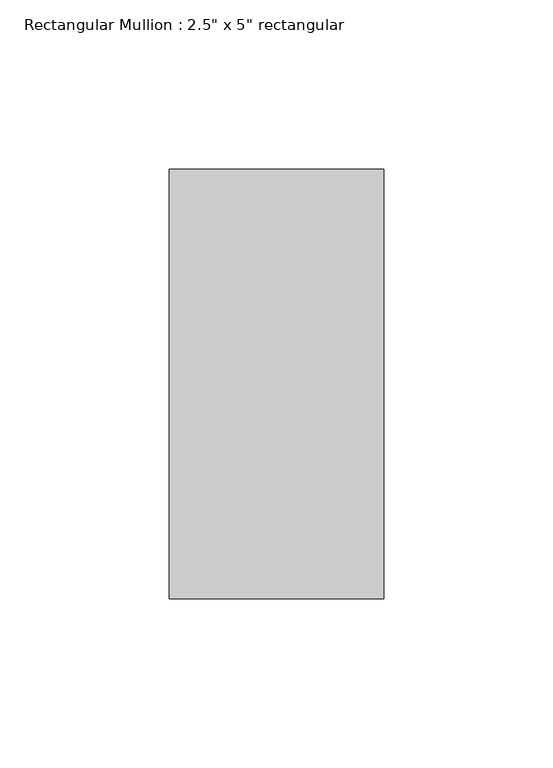
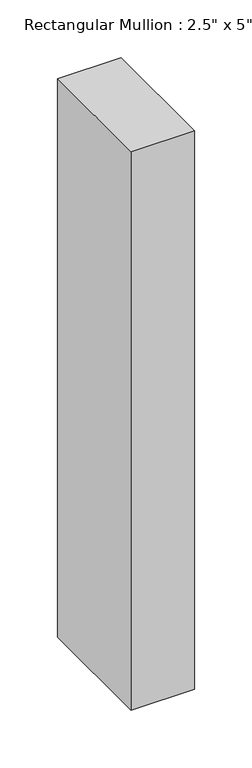
"""IFC4 building model written with IfcOpenShell, lengths in millimetres: member geometry."""

from ifc_helpers import new_model, si_unit, frame, origin, place, context, project, spatial, polyline, outline, extrude, source, transform, mapped, element, save


def member_e5d39754(model_context):
    return source(origin(), model_context, "Body", "SweptSolid", [
        extrude(outline(polyline([(0.0, 63.5), (0.0, -63.5), (-63.5, -63.5), (-63.5, 63.5), (0.0, 63.5)])), frame((0.0, 0.0, -590.55), z_axis=(0.0, 0.0, 1.0), x_axis=(1.0, 0.0, 0.0)), (0.0, 0.0, 1.0), 590.55),
    ])


if __name__ == "__main__":
    model = new_model("IFC4")
    model_context = context("Model", 3, world=origin())
    ifc_project = project(units=[si_unit("LENGTHUNIT", "METRE", prefix="MILLI")], contexts=[model_context])
    site = spatial("IfcSite", under=ifc_project)
    building = spatial("IfcBuilding", under=site)
    placement = place(None, origin())
    member_shape = member_e5d39754(model_context)
    element("IfcMember", 1, ObjectType="Rectangular Mullion : 2.5\" x 5\" rectangular", at=placement, inside=building, context=model_context, shape_type="MappedRepresentation", body=[
        mapped(member_shape, transform((0.0, 0.0, 0.0), x_axis=(1.0, 0.0, 0.0), y_axis=(0.0, 1.0, 0.0), z_axis=(0.0, 0.0, 1.0))),
    ])
    save(model, "model.ifc")

# Revit data of these elements
# Type "Rectangular Mullion : 2.5\" x 5\" rectangular"
#   built-in parameter 1007304 = 0.416667 (stored number, unit not read)
#   built-in parameter 1007301 = 0.104167 (stored number, unit not read)
#   built-in parameter 1007300 = 0.104167 (stored number, unit not read)
# Element 1 (IfcMember, "Rectangular Mullion : 2.5\" x 5\" rectangular")
#   Materials on its faces: "Aluminum"
# Materials
#   "Aluminum": class "Metal", colour RGB 247 247 247, transparency 0, Description = "Aluminum 6061", Cost = 0
